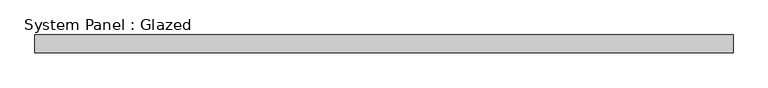
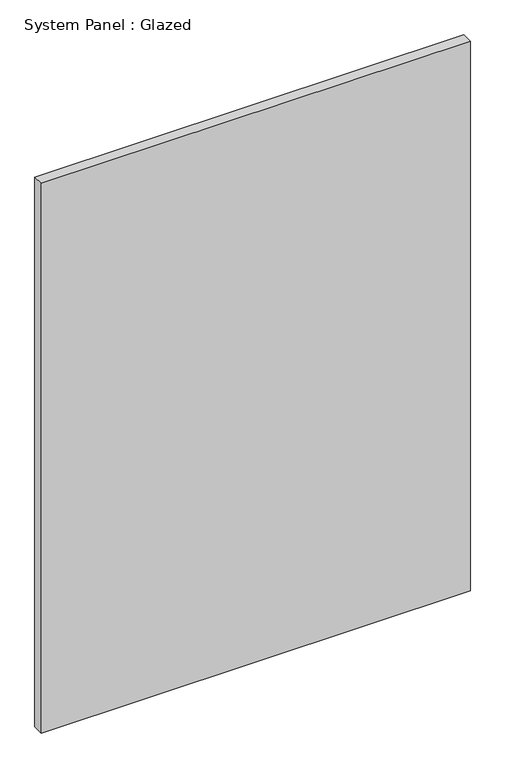
"""IFC4 building model written with IfcOpenShell, lengths in millimetres: plate geometry, System Panel : Glazed."""

from ifc_helpers import new_model, si_unit, origin, origin_with_axes, place, context, project, spatial, polyline, outline, extrude, source, transform, mapped, element, save


def system_panel_glazed_9cc9ac89(model_context):
    return source(origin(), model_context, "Body", "SweptSolid", [
        extrude(outline(polyline([(502.57075, 19.05), (-502.57075, 19.05), (-502.57075, 44.45), (502.57075, 44.45), (502.57075, 19.05)])), origin_with_axes(), (0.0, 0.0, 1.0), 1360.7415),
    ])


if __name__ == "__main__":
    model = new_model("IFC4")
    model_context = context("Model", 3, world=origin())
    ifc_project = project(units=[si_unit("LENGTHUNIT", "METRE", prefix="MILLI")], contexts=[model_context])
    site = spatial("IfcSite", under=ifc_project)
    building = spatial("IfcBuilding", under=site)
    placement = place(None, origin())
    system_panel_glazed_shape = system_panel_glazed_9cc9ac89(model_context)
    element("IfcPlate", 1, ObjectType="System Panel : Glazed", at=placement, inside=building, context=model_context, shape_type="MappedRepresentation", body=[
        mapped(system_panel_glazed_shape, transform((0.0, 0.0, 0.0), x_axis=(1.0, 0.0, 0.0), y_axis=(0.0, 1.0, 0.0), z_axis=(0.0, 0.0, 1.0))),
    ])
    save(model, "model.ifc")

# Revit data of these elements
# Type "System Panel : Glazed"
#   Construction Type Id = "GSP4R"
#   Analytic Construction = "1/8 in Pilkington single glazing"
#   Visual Light Transmittance = 0.9
#   Solar Heat Gain Coefficient = 0.86
#   Heat Transfer Coefficient (U) = 1.18115 BTU/(h·ft²·°F)
#   Define Thermal Properties by = 1
# Element 1 (IfcPlate, "System Panel : Glazed")
#   Materials on its faces: "Glass"
# Materials
#   "Glass": class "Glass", colour RGB 0 128 192, transparency 0.75, Description = "Soda Lime Glass", Cost = 0
